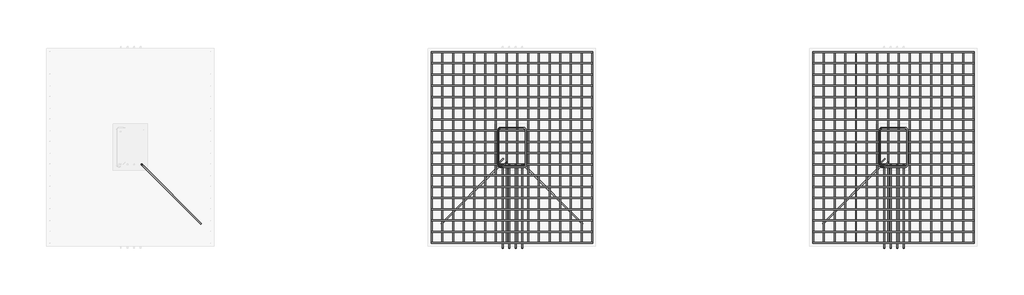
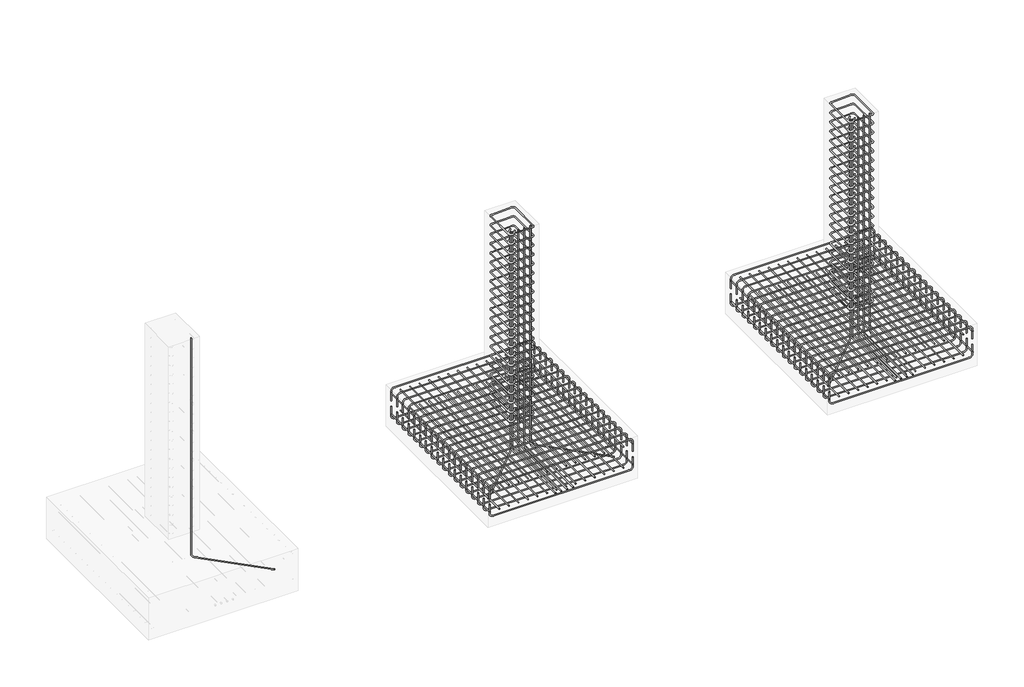
# One storey, part 7 of 33: 16 reinforcing bars.
"""IFC4 building model written with IfcOpenShell, lengths in millimetres."""

from ifc_helpers import new_model, si_unit, point, frame, origin, place, context, project, spatial, polyline, circle_curve, trimmed, segment, composite_curve, source, transform, mapped, element, save
from ifc_brep_helpers import swept_disk

model = new_model("IFC4")

# Units and contexts
model_context = context("Model", 3, world=origin())
ifc_project = project(units=[si_unit("LENGTHUNIT", "METRE", prefix="MILLI")], contexts=[model_context])

# Site, building, storey
site = spatial("IfcSite", under=ifc_project)
building = spatial("IfcBuilding", under=site)
storey = spatial("IfcBuildingStorey", under=building, Elevation=-3000.0)

# Reinforcing bars
placement = place(None, origin())
reinforcing_bar_shape = source(origin(), model_context, "Body", "SolidModel", [
    swept_disk(composite_curve([segment(polyline([(9306.5357258, -7044.0608134, -3240.0), (9306.5357258, -7044.0608134, -3092.7)]), True, "CONTINUOUS"), segment(trimmed(circle_curve(frame((9352.8857258, -7044.0608134, -3092.7), z_axis=(0.0, 1.0, 0.0), x_axis=(-46.350000000000364, 0.0, 0.0)), 46.35), [point((9306.5357258, -7044.0608134, -3092.7))], [point((9352.8857258, -7044.0608134, -3046.35))], True, "CARTESIAN"), True, "CONTINUOUS"), segment(polyline([(9352.8857258, -7044.0608134, -3046.35), (11367.4857258, -7044.0608134, -3046.35)]), True, "CONTINUOUS"), segment(trimmed(circle_curve(frame((11367.4857258, -7044.0608134, -3092.7), z_axis=(0.0, 1.0, 0.0), x_axis=(0.0, 0.0, 46.34999999999991)), 46.35), [point((11367.4857258, -7044.0608134, -3046.35))], [point((11413.8357258, -7044.0608134, -3092.7))], True, "CARTESIAN"), True, "CONTINUOUS"), segment(polyline([(11413.8357258, -7044.0608134, -3092.7), (11413.8357258, -7044.0608134, -3240.0)]), True, "CONTINUOUS")], self_intersect=False), 6.35),
])
element("IfcReinforcingBar", 1, at=placement, inside=storey, context=model_context, shape_type="MappedRepresentation", body=[
    mapped(reinforcing_bar_shape, transform((0.0, 0.0, 0.0), x_axis=(1.0, 0.0, 0.0), y_axis=(0.0, 1.0, 0.0), z_axis=(0.0, 0.0, 1.0))),
    mapped(reinforcing_bar_shape, transform((0.0, -147.4882353, 0.0), x_axis=(1.0, 0.0, 0.0), y_axis=(0.0, 1.0, 0.0), z_axis=(0.0, 0.0, 1.0))),
    mapped(reinforcing_bar_shape, transform((0.0, -294.9764706, 0.0), x_axis=(1.0, 0.0, 0.0), y_axis=(0.0, 1.0, 0.0), z_axis=(0.0, 0.0, 1.0))),
    mapped(reinforcing_bar_shape, transform((0.0, -442.4647059, 0.0), x_axis=(1.0, 0.0, 0.0), y_axis=(0.0, 1.0, 0.0), z_axis=(0.0, 0.0, 1.0))),
    mapped(reinforcing_bar_shape, transform((0.0, -589.9529412, 0.0), x_axis=(1.0, 0.0, 0.0), y_axis=(0.0, 1.0, 0.0), z_axis=(0.0, 0.0, 1.0))),
    mapped(reinforcing_bar_shape, transform((0.0, -737.4411765, 0.0), x_axis=(1.0, 0.0, 0.0), y_axis=(0.0, 1.0, 0.0), z_axis=(0.0, 0.0, 1.0))),
    mapped(reinforcing_bar_shape, transform((0.0, -884.9294118, 0.0), x_axis=(1.0, 0.0, 0.0), y_axis=(0.0, 1.0, 0.0), z_axis=(0.0, 0.0, 1.0))),
    mapped(reinforcing_bar_shape, transform((0.0, -1032.4176471, 0.0), x_axis=(1.0, 0.0, 0.0), y_axis=(0.0, 1.0, 0.0), z_axis=(0.0, 0.0, 1.0))),
    mapped(reinforcing_bar_shape, transform((0.0, -1179.9058824, 0.0), x_axis=(1.0, 0.0, 0.0), y_axis=(0.0, 1.0, 0.0), z_axis=(0.0, 0.0, 1.0))),
    mapped(reinforcing_bar_shape, transform((0.0, -1327.3941176, 0.0), x_axis=(1.0, 0.0, 0.0), y_axis=(0.0, 1.0, 0.0), z_axis=(0.0, 0.0, 1.0))),
    mapped(reinforcing_bar_shape, transform((0.0, -1474.8823529, 0.0), x_axis=(1.0, 0.0, 0.0), y_axis=(0.0, 1.0, 0.0), z_axis=(0.0, 0.0, 1.0))),
    mapped(reinforcing_bar_shape, transform((0.0, -1622.3705882, 0.0), x_axis=(1.0, 0.0, 0.0), y_axis=(0.0, 1.0, 0.0), z_axis=(0.0, 0.0, 1.0))),
    mapped(reinforcing_bar_shape, transform((0.0, -1769.8588235, 0.0), x_axis=(1.0, 0.0, 0.0), y_axis=(0.0, 1.0, 0.0), z_axis=(0.0, 0.0, 1.0))),
    mapped(reinforcing_bar_shape, transform((0.0, -1917.3470588, 0.0), x_axis=(1.0, 0.0, 0.0), y_axis=(0.0, 1.0, 0.0), z_axis=(0.0, 0.0, 1.0))),
    mapped(reinforcing_bar_shape, transform((0.0, -2064.8352941, 0.0), x_axis=(1.0, 0.0, 0.0), y_axis=(0.0, 1.0, 0.0), z_axis=(0.0, 0.0, 1.0))),
    mapped(reinforcing_bar_shape, transform((0.0, -2212.3235294, 0.0), x_axis=(1.0, 0.0, 0.0), y_axis=(0.0, 1.0, 0.0), z_axis=(0.0, 0.0, 1.0))),
    mapped(reinforcing_bar_shape, transform((0.0, -2359.8117647, 0.0), x_axis=(1.0, 0.0, 0.0), y_axis=(0.0, 1.0, 0.0), z_axis=(0.0, 0.0, 1.0))),
    mapped(reinforcing_bar_shape, transform((0.0, -2507.3, 0.0), x_axis=(1.0, 0.0, 0.0), y_axis=(0.0, 1.0, 0.0), z_axis=(0.0, 0.0, 1.0))),
])
reinforcing_bar_2_shape = source(origin(), model_context, "Body", "SolidModel", [
    swept_disk(composite_curve([segment(polyline([(11413.8357258, -7044.0608134, -3330.080452), (11413.8357258, -7044.0608134, -3477.380452)]), True, "CONTINUOUS"), segment(trimmed(circle_curve(frame((11367.4857258, -7044.0608134, -3477.380452), z_axis=(0.0, 1.0, 0.0), x_axis=(46.350000000000364, 0.0, 0.0)), 46.35), [point((11413.8357258, -7044.0608134, -3477.380452))], [point((11367.4857258, -7044.0608134, -3523.730452))], True, "CARTESIAN"), True, "CONTINUOUS"), segment(polyline([(11367.4857258, -7044.0608134, -3523.730452), (9352.8857258, -7044.0608134, -3523.730452)]), True, "CONTINUOUS"), segment(trimmed(circle_curve(frame((9352.8857258, -7044.0608134, -3477.380452), z_axis=(0.0, 1.0, 0.0), x_axis=(0.0, 0.0, -46.34999999999991)), 46.35), [point((9352.8857258, -7044.0608134, -3523.730452))], [point((9306.5357258, -7044.0608134, -3477.380452))], True, "CARTESIAN"), True, "CONTINUOUS"), segment(polyline([(9306.5357258, -7044.0608134, -3477.380452), (9306.5357258, -7044.0608134, -3330.080452)]), True, "CONTINUOUS")], self_intersect=False), 6.35),
])
element("IfcReinforcingBar", 2, at=placement, inside=storey, context=model_context, shape_type="MappedRepresentation", body=[
    mapped(reinforcing_bar_2_shape, transform((0.0, 0.0, 0.0), x_axis=(1.0, 0.0, 0.0), y_axis=(0.0, 1.0, 0.0), z_axis=(0.0, 0.0, 1.0))),
    mapped(reinforcing_bar_2_shape, transform((0.0, -147.4882353, 0.0), x_axis=(1.0, 0.0, 0.0), y_axis=(0.0, 1.0, 0.0), z_axis=(0.0, 0.0, 1.0))),
    mapped(reinforcing_bar_2_shape, transform((0.0, -294.9764706, 0.0), x_axis=(1.0, 0.0, 0.0), y_axis=(0.0, 1.0, 0.0), z_axis=(0.0, 0.0, 1.0))),
    mapped(reinforcing_bar_2_shape, transform((0.0, -442.4647059, 0.0), x_axis=(1.0, 0.0, 0.0), y_axis=(0.0, 1.0, 0.0), z_axis=(0.0, 0.0, 1.0))),
    mapped(reinforcing_bar_2_shape, transform((0.0, -589.9529412, 0.0), x_axis=(1.0, 0.0, 0.0), y_axis=(0.0, 1.0, 0.0), z_axis=(0.0, 0.0, 1.0))),
    mapped(reinforcing_bar_2_shape, transform((0.0, -737.4411765, 0.0), x_axis=(1.0, 0.0, 0.0), y_axis=(0.0, 1.0, 0.0), z_axis=(0.0, 0.0, 1.0))),
    mapped(reinforcing_bar_2_shape, transform((0.0, -884.9294118, 0.0), x_axis=(1.0, 0.0, 0.0), y_axis=(0.0, 1.0, 0.0), z_axis=(0.0, 0.0, 1.0))),
    mapped(reinforcing_bar_2_shape, transform((0.0, -1032.4176471, 0.0), x_axis=(1.0, 0.0, 0.0), y_axis=(0.0, 1.0, 0.0), z_axis=(0.0, 0.0, 1.0))),
    mapped(reinforcing_bar_2_shape, transform((0.0, -1179.9058824, 0.0), x_axis=(1.0, 0.0, 0.0), y_axis=(0.0, 1.0, 0.0), z_axis=(0.0, 0.0, 1.0))),
    mapped(reinforcing_bar_2_shape, transform((0.0, -1327.3941176, 0.0), x_axis=(1.0, 0.0, 0.0), y_axis=(0.0, 1.0, 0.0), z_axis=(0.0, 0.0, 1.0))),
    mapped(reinforcing_bar_2_shape, transform((0.0, -1474.8823529, 0.0), x_axis=(1.0, 0.0, 0.0), y_axis=(0.0, 1.0, 0.0), z_axis=(0.0, 0.0, 1.0))),
    mapped(reinforcing_bar_2_shape, transform((0.0, -1622.3705882, 0.0), x_axis=(1.0, 0.0, 0.0), y_axis=(0.0, 1.0, 0.0), z_axis=(0.0, 0.0, 1.0))),
    mapped(reinforcing_bar_2_shape, transform((0.0, -1769.8588235, 0.0), x_axis=(1.0, 0.0, 0.0), y_axis=(0.0, 1.0, 0.0), z_axis=(0.0, 0.0, 1.0))),
    mapped(reinforcing_bar_2_shape, transform((0.0, -1917.3470588, 0.0), x_axis=(1.0, 0.0, 0.0), y_axis=(0.0, 1.0, 0.0), z_axis=(0.0, 0.0, 1.0))),
    mapped(reinforcing_bar_2_shape, transform((0.0, -2064.8352941, 0.0), x_axis=(1.0, 0.0, 0.0), y_axis=(0.0, 1.0, 0.0), z_axis=(0.0, 0.0, 1.0))),
    mapped(reinforcing_bar_2_shape, transform((0.0, -2212.3235294, 0.0), x_axis=(1.0, 0.0, 0.0), y_axis=(0.0, 1.0, 0.0), z_axis=(0.0, 0.0, 1.0))),
    mapped(reinforcing_bar_2_shape, transform((0.0, -2359.8117647, 0.0), x_axis=(1.0, 0.0, 0.0), y_axis=(0.0, 1.0, 0.0), z_axis=(0.0, 0.0, 1.0))),
    mapped(reinforcing_bar_2_shape, transform((0.0, -2507.3, 0.0), x_axis=(1.0, 0.0, 0.0), y_axis=(0.0, 1.0, 0.0), z_axis=(0.0, 0.0, 1.0))),
])
reinforcing_bar_3_shape = source(origin(), model_context, "Body", "SolidModel", [
    swept_disk(composite_curve([segment(polyline([(11413.8357258, -9557.7108134, -3447.8614173), (11413.8357258, -7037.7108134, -3447.8614173)]), True, "CONTINUOUS")], self_intersect=False), 6.35),
])
element("IfcReinforcingBar", 3, at=placement, inside=storey, context=model_context, shape_type="MappedRepresentation", body=[
    mapped(reinforcing_bar_3_shape, transform((0.0, 0.0, 0.0), x_axis=(1.0, 0.0, 0.0), y_axis=(0.0, 1.0, 0.0), z_axis=(0.0, 0.0, 1.0))),
    mapped(reinforcing_bar_3_shape, transform((-140.4866667, 0.0, 0.0), x_axis=(1.0, 0.0, 0.0), y_axis=(0.0, 1.0, 0.0), z_axis=(0.0, 0.0, 1.0))),
    mapped(reinforcing_bar_3_shape, transform((-280.9733333, 0.0, 0.0), x_axis=(1.0, 0.0, 0.0), y_axis=(0.0, 1.0, 0.0), z_axis=(0.0, 0.0, 1.0))),
    mapped(reinforcing_bar_3_shape, transform((-421.46, 0.0, 0.0), x_axis=(1.0, 0.0, 0.0), y_axis=(0.0, 1.0, 0.0), z_axis=(0.0, 0.0, 1.0))),
    mapped(reinforcing_bar_3_shape, transform((-561.9466667, 0.0, 0.0), x_axis=(1.0, 0.0, 0.0), y_axis=(0.0, 1.0, 0.0), z_axis=(0.0, 0.0, 1.0))),
    mapped(reinforcing_bar_3_shape, transform((-702.4333333, 0.0, 0.0), x_axis=(1.0, 0.0, 0.0), y_axis=(0.0, 1.0, 0.0), z_axis=(0.0, 0.0, 1.0))),
    mapped(reinforcing_bar_3_shape, transform((-842.92, 0.0, 0.0), x_axis=(1.0, 0.0, 0.0), y_axis=(0.0, 1.0, 0.0), z_axis=(0.0, 0.0, 1.0))),
    mapped(reinforcing_bar_3_shape, transform((-983.4066667, 0.0, 0.0), x_axis=(1.0, 0.0, 0.0), y_axis=(0.0, 1.0, 0.0), z_axis=(0.0, 0.0, 1.0))),
    mapped(reinforcing_bar_3_shape, transform((-1123.8933333, 0.0, 0.0), x_axis=(1.0, 0.0, 0.0), y_axis=(0.0, 1.0, 0.0), z_axis=(0.0, 0.0, 1.0))),
    mapped(reinforcing_bar_3_shape, transform((-1264.38, 0.0, 0.0), x_axis=(1.0, 0.0, 0.0), y_axis=(0.0, 1.0, 0.0), z_axis=(0.0, 0.0, 1.0))),
    mapped(reinforcing_bar_3_shape, transform((-1404.8666667, 0.0, 0.0), x_axis=(1.0, 0.0, 0.0), y_axis=(0.0, 1.0, 0.0), z_axis=(0.0, 0.0, 1.0))),
    mapped(reinforcing_bar_3_shape, transform((-1545.3533333, 0.0, 0.0), x_axis=(1.0, 0.0, 0.0), y_axis=(0.0, 1.0, 0.0), z_axis=(0.0, 0.0, 1.0))),
    mapped(reinforcing_bar_3_shape, transform((-1685.84, 0.0, 0.0), x_axis=(1.0, 0.0, 0.0), y_axis=(0.0, 1.0, 0.0), z_axis=(0.0, 0.0, 1.0))),
    mapped(reinforcing_bar_3_shape, transform((-1826.3266667, 0.0, 0.0), x_axis=(1.0, 0.0, 0.0), y_axis=(0.0, 1.0, 0.0), z_axis=(0.0, 0.0, 1.0))),
    mapped(reinforcing_bar_3_shape, transform((-1966.8133333, 0.0, 0.0), x_axis=(1.0, 0.0, 0.0), y_axis=(0.0, 1.0, 0.0), z_axis=(0.0, 0.0, 1.0))),
    mapped(reinforcing_bar_3_shape, transform((-2107.3, 0.0, 0.0), x_axis=(1.0, 0.0, 0.0), y_axis=(0.0, 1.0, 0.0), z_axis=(0.0, 0.0, 1.0))),
])
reinforcing_bar_4_shape = source(origin(), model_context, "Body", "SolidModel", [
    swept_disk(composite_curve([segment(polyline([(9306.5357258, -9557.7108134, -3122.7084113), (9306.5357258, -7037.7108134, -3122.7084113)]), True, "CONTINUOUS")], self_intersect=False), 6.35),
])
element("IfcReinforcingBar", 4, at=placement, inside=storey, context=model_context, shape_type="MappedRepresentation", body=[
    mapped(reinforcing_bar_4_shape, transform((0.0, 0.0, 0.0), x_axis=(1.0, 0.0, 0.0), y_axis=(0.0, 1.0, 0.0), z_axis=(0.0, 0.0, 1.0))),
    mapped(reinforcing_bar_4_shape, transform((140.4866667, 0.0, 0.0), x_axis=(1.0, 0.0, 0.0), y_axis=(0.0, 1.0, 0.0), z_axis=(0.0, 0.0, 1.0))),
    mapped(reinforcing_bar_4_shape, transform((280.9733333, 0.0, 0.0), x_axis=(1.0, 0.0, 0.0), y_axis=(0.0, 1.0, 0.0), z_axis=(0.0, 0.0, 1.0))),
    mapped(reinforcing_bar_4_shape, transform((421.46, 0.0, 0.0), x_axis=(1.0, 0.0, 0.0), y_axis=(0.0, 1.0, 0.0), z_axis=(0.0, 0.0, 1.0))),
    mapped(reinforcing_bar_4_shape, transform((561.9466667, 0.0, 0.0), x_axis=(1.0, 0.0, 0.0), y_axis=(0.0, 1.0, 0.0), z_axis=(0.0, 0.0, 1.0))),
    mapped(reinforcing_bar_4_shape, transform((702.4333333, 0.0, 0.0), x_axis=(1.0, 0.0, 0.0), y_axis=(0.0, 1.0, 0.0), z_axis=(0.0, 0.0, 1.0))),
    mapped(reinforcing_bar_4_shape, transform((842.92, 0.0, 0.0), x_axis=(1.0, 0.0, 0.0), y_axis=(0.0, 1.0, 0.0), z_axis=(0.0, 0.0, 1.0))),
    mapped(reinforcing_bar_4_shape, transform((983.4066667, 0.0, 0.0), x_axis=(1.0, 0.0, 0.0), y_axis=(0.0, 1.0, 0.0), z_axis=(0.0, 0.0, 1.0))),
    mapped(reinforcing_bar_4_shape, transform((1123.8933333, 0.0, 0.0), x_axis=(1.0, 0.0, 0.0), y_axis=(0.0, 1.0, 0.0), z_axis=(0.0, 0.0, 1.0))),
    mapped(reinforcing_bar_4_shape, transform((1264.38, 0.0, 0.0), x_axis=(1.0, 0.0, 0.0), y_axis=(0.0, 1.0, 0.0), z_axis=(0.0, 0.0, 1.0))),
    mapped(reinforcing_bar_4_shape, transform((1404.8666667, 0.0, 0.0), x_axis=(1.0, 0.0, 0.0), y_axis=(0.0, 1.0, 0.0), z_axis=(0.0, 0.0, 1.0))),
    mapped(reinforcing_bar_4_shape, transform((1545.3533333, 0.0, 0.0), x_axis=(1.0, 0.0, 0.0), y_axis=(0.0, 1.0, 0.0), z_axis=(0.0, 0.0, 1.0))),
    mapped(reinforcing_bar_4_shape, transform((1685.84, 0.0, 0.0), x_axis=(1.0, 0.0, 0.0), y_axis=(0.0, 1.0, 0.0), z_axis=(0.0, 0.0, 1.0))),
    mapped(reinforcing_bar_4_shape, transform((1826.3266667, 0.0, 0.0), x_axis=(1.0, 0.0, 0.0), y_axis=(0.0, 1.0, 0.0), z_axis=(0.0, 0.0, 1.0))),
    mapped(reinforcing_bar_4_shape, transform((1966.8133333, 0.0, 0.0), x_axis=(1.0, 0.0, 0.0), y_axis=(0.0, 1.0, 0.0), z_axis=(0.0, 0.0, 1.0))),
    mapped(reinforcing_bar_4_shape, transform((2107.3, 0.0, 0.0), x_axis=(1.0, 0.0, 0.0), y_axis=(0.0, 1.0, 0.0), z_axis=(0.0, 0.0, 1.0))),
])
reinforcing_bar_5_shape = source(origin(), model_context, "Body", "SolidModel", [
    swept_disk(composite_curve([segment(polyline([(4306.5357258, -7044.0608134, -3240.0), (4306.5357258, -7044.0608134, -3092.7)]), True, "CONTINUOUS"), segment(trimmed(circle_curve(frame((4352.8857258, -7044.0608134, -3092.7), z_axis=(0.0, 1.0, 0.0), x_axis=(-46.349999999999454, 0.0, 0.0)), 46.35), [point((4306.5357258, -7044.0608134, -3092.7))], [point((4352.8857258, -7044.0608134, -3046.35))], True, "CARTESIAN"), True, "CONTINUOUS"), segment(polyline([(4352.8857258, -7044.0608134, -3046.35), (6367.4857258, -7044.0608134, -3046.35)]), True, "CONTINUOUS"), segment(trimmed(circle_curve(frame((6367.4857258, -7044.0608134, -3092.7), z_axis=(0.0, 1.0, 0.0), x_axis=(0.0, 0.0, 46.34999999999991)), 46.35), [point((6367.4857258, -7044.0608134, -3046.35))], [point((6413.8357258, -7044.0608134, -3092.7))], True, "CARTESIAN"), True, "CONTINUOUS"), segment(polyline([(6413.8357258, -7044.0608134, -3092.7), (6413.8357258, -7044.0608134, -3240.0)]), True, "CONTINUOUS")], self_intersect=False), 6.35),
])
element("IfcReinforcingBar", 5, at=placement, inside=storey, context=model_context, shape_type="MappedRepresentation", body=[
    mapped(reinforcing_bar_5_shape, transform((0.0, 0.0, 0.0), x_axis=(1.0, 0.0, 0.0), y_axis=(0.0, 1.0, 0.0), z_axis=(0.0, 0.0, 1.0))),
    mapped(reinforcing_bar_5_shape, transform((0.0, -147.4882353, 0.0), x_axis=(1.0, 0.0, 0.0), y_axis=(0.0, 1.0, 0.0), z_axis=(0.0, 0.0, 1.0))),
    mapped(reinforcing_bar_5_shape, transform((0.0, -294.9764706, 0.0), x_axis=(1.0, 0.0, 0.0), y_axis=(0.0, 1.0, 0.0), z_axis=(0.0, 0.0, 1.0))),
    mapped(reinforcing_bar_5_shape, transform((0.0, -442.4647059, 0.0), x_axis=(1.0, 0.0, 0.0), y_axis=(0.0, 1.0, 0.0), z_axis=(0.0, 0.0, 1.0))),
    mapped(reinforcing_bar_5_shape, transform((0.0, -589.9529412, 0.0), x_axis=(1.0, 0.0, 0.0), y_axis=(0.0, 1.0, 0.0), z_axis=(0.0, 0.0, 1.0))),
    mapped(reinforcing_bar_5_shape, transform((0.0, -737.4411765, 0.0), x_axis=(1.0, 0.0, 0.0), y_axis=(0.0, 1.0, 0.0), z_axis=(0.0, 0.0, 1.0))),
    mapped(reinforcing_bar_5_shape, transform((0.0, -884.9294118, 0.0), x_axis=(1.0, 0.0, 0.0), y_axis=(0.0, 1.0, 0.0), z_axis=(0.0, 0.0, 1.0))),
    mapped(reinforcing_bar_5_shape, transform((0.0, -1032.4176471, 0.0), x_axis=(1.0, 0.0, 0.0), y_axis=(0.0, 1.0, 0.0), z_axis=(0.0, 0.0, 1.0))),
    mapped(reinforcing_bar_5_shape, transform((0.0, -1179.9058824, 0.0), x_axis=(1.0, 0.0, 0.0), y_axis=(0.0, 1.0, 0.0), z_axis=(0.0, 0.0, 1.0))),
    mapped(reinforcing_bar_5_shape, transform((0.0, -1327.3941176, 0.0), x_axis=(1.0, 0.0, 0.0), y_axis=(0.0, 1.0, 0.0), z_axis=(0.0, 0.0, 1.0))),
    mapped(reinforcing_bar_5_shape, transform((0.0, -1474.8823529, 0.0), x_axis=(1.0, 0.0, 0.0), y_axis=(0.0, 1.0, 0.0), z_axis=(0.0, 0.0, 1.0))),
    mapped(reinforcing_bar_5_shape, transform((0.0, -1622.3705882, 0.0), x_axis=(1.0, 0.0, 0.0), y_axis=(0.0, 1.0, 0.0), z_axis=(0.0, 0.0, 1.0))),
    mapped(reinforcing_bar_5_shape, transform((0.0, -1769.8588235, 0.0), x_axis=(1.0, 0.0, 0.0), y_axis=(0.0, 1.0, 0.0), z_axis=(0.0, 0.0, 1.0))),
    mapped(reinforcing_bar_5_shape, transform((0.0, -1917.3470588, 0.0), x_axis=(1.0, 0.0, 0.0), y_axis=(0.0, 1.0, 0.0), z_axis=(0.0, 0.0, 1.0))),
    mapped(reinforcing_bar_5_shape, transform((0.0, -2064.8352941, 0.0), x_axis=(1.0, 0.0, 0.0), y_axis=(0.0, 1.0, 0.0), z_axis=(0.0, 0.0, 1.0))),
    mapped(reinforcing_bar_5_shape, transform((0.0, -2212.3235294, 0.0), x_axis=(1.0, 0.0, 0.0), y_axis=(0.0, 1.0, 0.0), z_axis=(0.0, 0.0, 1.0))),
    mapped(reinforcing_bar_5_shape, transform((0.0, -2359.8117647, 0.0), x_axis=(1.0, 0.0, 0.0), y_axis=(0.0, 1.0, 0.0), z_axis=(0.0, 0.0, 1.0))),
    mapped(reinforcing_bar_5_shape, transform((0.0, -2507.3, 0.0), x_axis=(1.0, 0.0, 0.0), y_axis=(0.0, 1.0, 0.0), z_axis=(0.0, 0.0, 1.0))),
])
reinforcing_bar_6_shape = source(origin(), model_context, "Body", "SolidModel", [
    swept_disk(composite_curve([segment(polyline([(6413.8357258, -7044.0608134, -3330.080452), (6413.8357258, -7044.0608134, -3477.380452)]), True, "CONTINUOUS"), segment(trimmed(circle_curve(frame((6367.4857258, -7044.0608134, -3477.380452), z_axis=(0.0, 1.0, 0.0), x_axis=(46.349999999999454, 0.0, 0.0)), 46.35), [point((6413.8357258, -7044.0608134, -3477.380452))], [point((6367.4857258, -7044.0608134, -3523.730452))], True, "CARTESIAN"), True, "CONTINUOUS"), segment(polyline([(6367.4857258, -7044.0608134, -3523.730452), (4352.8857258, -7044.0608134, -3523.730452)]), True, "CONTINUOUS"), segment(trimmed(circle_curve(frame((4352.8857258, -7044.0608134, -3477.380452), z_axis=(0.0, 1.0, 0.0), x_axis=(0.0, 0.0, -46.34999999999991)), 46.35), [point((4352.8857258, -7044.0608134, -3523.730452))], [point((4306.5357258, -7044.0608134, -3477.380452))], True, "CARTESIAN"), True, "CONTINUOUS"), segment(polyline([(4306.5357258, -7044.0608134, -3477.380452), (4306.5357258, -7044.0608134, -3330.080452)]), True, "CONTINUOUS")], self_intersect=False), 6.35),
])
element("IfcReinforcingBar", 6, at=placement, inside=storey, context=model_context, shape_type="MappedRepresentation", body=[
    mapped(reinforcing_bar_6_shape, transform((0.0, 0.0, 0.0), x_axis=(1.0, 0.0, 0.0), y_axis=(0.0, 1.0, 0.0), z_axis=(0.0, 0.0, 1.0))),
    mapped(reinforcing_bar_6_shape, transform((0.0, -147.4882353, 0.0), x_axis=(1.0, 0.0, 0.0), y_axis=(0.0, 1.0, 0.0), z_axis=(0.0, 0.0, 1.0))),
    mapped(reinforcing_bar_6_shape, transform((0.0, -294.9764706, 0.0), x_axis=(1.0, 0.0, 0.0), y_axis=(0.0, 1.0, 0.0), z_axis=(0.0, 0.0, 1.0))),
    mapped(reinforcing_bar_6_shape, transform((0.0, -442.4647059, 0.0), x_axis=(1.0, 0.0, 0.0), y_axis=(0.0, 1.0, 0.0), z_axis=(0.0, 0.0, 1.0))),
    mapped(reinforcing_bar_6_shape, transform((0.0, -589.9529412, 0.0), x_axis=(1.0, 0.0, 0.0), y_axis=(0.0, 1.0, 0.0), z_axis=(0.0, 0.0, 1.0))),
    mapped(reinforcing_bar_6_shape, transform((0.0, -737.4411765, 0.0), x_axis=(1.0, 0.0, 0.0), y_axis=(0.0, 1.0, 0.0), z_axis=(0.0, 0.0, 1.0))),
    mapped(reinforcing_bar_6_shape, transform((0.0, -884.9294118, 0.0), x_axis=(1.0, 0.0, 0.0), y_axis=(0.0, 1.0, 0.0), z_axis=(0.0, 0.0, 1.0))),
    mapped(reinforcing_bar_6_shape, transform((0.0, -1032.4176471, 0.0), x_axis=(1.0, 0.0, 0.0), y_axis=(0.0, 1.0, 0.0), z_axis=(0.0, 0.0, 1.0))),
    mapped(reinforcing_bar_6_shape, transform((0.0, -1179.9058824, 0.0), x_axis=(1.0, 0.0, 0.0), y_axis=(0.0, 1.0, 0.0), z_axis=(0.0, 0.0, 1.0))),
    mapped(reinforcing_bar_6_shape, transform((0.0, -1327.3941176, 0.0), x_axis=(1.0, 0.0, 0.0), y_axis=(0.0, 1.0, 0.0), z_axis=(0.0, 0.0, 1.0))),
    mapped(reinforcing_bar_6_shape, transform((0.0, -1474.8823529, 0.0), x_axis=(1.0, 0.0, 0.0), y_axis=(0.0, 1.0, 0.0), z_axis=(0.0, 0.0, 1.0))),
    mapped(reinforcing_bar_6_shape, transform((0.0, -1622.3705882, 0.0), x_axis=(1.0, 0.0, 0.0), y_axis=(0.0, 1.0, 0.0), z_axis=(0.0, 0.0, 1.0))),
    mapped(reinforcing_bar_6_shape, transform((0.0, -1769.8588235, 0.0), x_axis=(1.0, 0.0, 0.0), y_axis=(0.0, 1.0, 0.0), z_axis=(0.0, 0.0, 1.0))),
    mapped(reinforcing_bar_6_shape, transform((0.0, -1917.3470588, 0.0), x_axis=(1.0, 0.0, 0.0), y_axis=(0.0, 1.0, 0.0), z_axis=(0.0, 0.0, 1.0))),
    mapped(reinforcing_bar_6_shape, transform((0.0, -2064.8352941, 0.0), x_axis=(1.0, 0.0, 0.0), y_axis=(0.0, 1.0, 0.0), z_axis=(0.0, 0.0, 1.0))),
    mapped(reinforcing_bar_6_shape, transform((0.0, -2212.3235294, 0.0), x_axis=(1.0, 0.0, 0.0), y_axis=(0.0, 1.0, 0.0), z_axis=(0.0, 0.0, 1.0))),
    mapped(reinforcing_bar_6_shape, transform((0.0, -2359.8117647, 0.0), x_axis=(1.0, 0.0, 0.0), y_axis=(0.0, 1.0, 0.0), z_axis=(0.0, 0.0, 1.0))),
    mapped(reinforcing_bar_6_shape, transform((0.0, -2507.3, 0.0), x_axis=(1.0, 0.0, 0.0), y_axis=(0.0, 1.0, 0.0), z_axis=(0.0, 0.0, 1.0))),
])
reinforcing_bar_7_shape = source(origin(), model_context, "Body", "SolidModel", [
    swept_disk(composite_curve([segment(polyline([(6413.8357258, -9557.7108134, -3447.8614173), (6413.8357258, -7037.7108134, -3447.8614173)]), True, "CONTINUOUS")], self_intersect=False), 6.35),
])
element("IfcReinforcingBar", 7, at=placement, inside=storey, context=model_context, shape_type="MappedRepresentation", body=[
    mapped(reinforcing_bar_7_shape, transform((0.0, 0.0, 0.0), x_axis=(1.0, 0.0, 0.0), y_axis=(0.0, 1.0, 0.0), z_axis=(0.0, 0.0, 1.0))),
    mapped(reinforcing_bar_7_shape, transform((-140.4866667, 0.0, 0.0), x_axis=(1.0, 0.0, 0.0), y_axis=(0.0, 1.0, 0.0), z_axis=(0.0, 0.0, 1.0))),
    mapped(reinforcing_bar_7_shape, transform((-280.9733333, 0.0, 0.0), x_axis=(1.0, 0.0, 0.0), y_axis=(0.0, 1.0, 0.0), z_axis=(0.0, 0.0, 1.0))),
    mapped(reinforcing_bar_7_shape, transform((-421.46, 0.0, 0.0), x_axis=(1.0, 0.0, 0.0), y_axis=(0.0, 1.0, 0.0), z_axis=(0.0, 0.0, 1.0))),
    mapped(reinforcing_bar_7_shape, transform((-561.9466667, 0.0, 0.0), x_axis=(1.0, 0.0, 0.0), y_axis=(0.0, 1.0, 0.0), z_axis=(0.0, 0.0, 1.0))),
    mapped(reinforcing_bar_7_shape, transform((-702.4333333, 0.0, 0.0), x_axis=(1.0, 0.0, 0.0), y_axis=(0.0, 1.0, 0.0), z_axis=(0.0, 0.0, 1.0))),
    mapped(reinforcing_bar_7_shape, transform((-842.92, 0.0, 0.0), x_axis=(1.0, 0.0, 0.0), y_axis=(0.0, 1.0, 0.0), z_axis=(0.0, 0.0, 1.0))),
    mapped(reinforcing_bar_7_shape, transform((-983.4066667, 0.0, 0.0), x_axis=(1.0, 0.0, 0.0), y_axis=(0.0, 1.0, 0.0), z_axis=(0.0, 0.0, 1.0))),
    mapped(reinforcing_bar_7_shape, transform((-1123.8933333, 0.0, 0.0), x_axis=(1.0, 0.0, 0.0), y_axis=(0.0, 1.0, 0.0), z_axis=(0.0, 0.0, 1.0))),
    mapped(reinforcing_bar_7_shape, transform((-1264.38, 0.0, 0.0), x_axis=(1.0, 0.0, 0.0), y_axis=(0.0, 1.0, 0.0), z_axis=(0.0, 0.0, 1.0))),
    mapped(reinforcing_bar_7_shape, transform((-1404.8666667, 0.0, 0.0), x_axis=(1.0, 0.0, 0.0), y_axis=(0.0, 1.0, 0.0), z_axis=(0.0, 0.0, 1.0))),
    mapped(reinforcing_bar_7_shape, transform((-1545.3533333, 0.0, 0.0), x_axis=(1.0, 0.0, 0.0), y_axis=(0.0, 1.0, 0.0), z_axis=(0.0, 0.0, 1.0))),
    mapped(reinforcing_bar_7_shape, transform((-1685.84, 0.0, 0.0), x_axis=(1.0, 0.0, 0.0), y_axis=(0.0, 1.0, 0.0), z_axis=(0.0, 0.0, 1.0))),
    mapped(reinforcing_bar_7_shape, transform((-1826.3266667, 0.0, 0.0), x_axis=(1.0, 0.0, 0.0), y_axis=(0.0, 1.0, 0.0), z_axis=(0.0, 0.0, 1.0))),
    mapped(reinforcing_bar_7_shape, transform((-1966.8133333, 0.0, 0.0), x_axis=(1.0, 0.0, 0.0), y_axis=(0.0, 1.0, 0.0), z_axis=(0.0, 0.0, 1.0))),
    mapped(reinforcing_bar_7_shape, transform((-2107.3, 0.0, 0.0), x_axis=(1.0, 0.0, 0.0), y_axis=(0.0, 1.0, 0.0), z_axis=(0.0, 0.0, 1.0))),
])
reinforcing_bar_8_shape = source(origin(), model_context, "Body", "SolidModel", [
    swept_disk(composite_curve([segment(polyline([(4306.5357258, -9557.7108134, -3122.7084113), (4306.5357258, -7037.7108134, -3122.7084113)]), True, "CONTINUOUS")], self_intersect=False), 6.35),
])
element("IfcReinforcingBar", 8, at=placement, inside=storey, context=model_context, shape_type="MappedRepresentation", body=[
    mapped(reinforcing_bar_8_shape, transform((0.0, 0.0, 0.0), x_axis=(1.0, 0.0, 0.0), y_axis=(0.0, 1.0, 0.0), z_axis=(0.0, 0.0, 1.0))),
    mapped(reinforcing_bar_8_shape, transform((140.4866667, 0.0, 0.0), x_axis=(1.0, 0.0, 0.0), y_axis=(0.0, 1.0, 0.0), z_axis=(0.0, 0.0, 1.0))),
    mapped(reinforcing_bar_8_shape, transform((280.9733333, 0.0, 0.0), x_axis=(1.0, 0.0, 0.0), y_axis=(0.0, 1.0, 0.0), z_axis=(0.0, 0.0, 1.0))),
    mapped(reinforcing_bar_8_shape, transform((421.46, 0.0, 0.0), x_axis=(1.0, 0.0, 0.0), y_axis=(0.0, 1.0, 0.0), z_axis=(0.0, 0.0, 1.0))),
    mapped(reinforcing_bar_8_shape, transform((561.9466667, 0.0, 0.0), x_axis=(1.0, 0.0, 0.0), y_axis=(0.0, 1.0, 0.0), z_axis=(0.0, 0.0, 1.0))),
    mapped(reinforcing_bar_8_shape, transform((702.4333333, 0.0, 0.0), x_axis=(1.0, 0.0, 0.0), y_axis=(0.0, 1.0, 0.0), z_axis=(0.0, 0.0, 1.0))),
    mapped(reinforcing_bar_8_shape, transform((842.92, 0.0, 0.0), x_axis=(1.0, 0.0, 0.0), y_axis=(0.0, 1.0, 0.0), z_axis=(0.0, 0.0, 1.0))),
    mapped(reinforcing_bar_8_shape, transform((983.4066667, 0.0, 0.0), x_axis=(1.0, 0.0, 0.0), y_axis=(0.0, 1.0, 0.0), z_axis=(0.0, 0.0, 1.0))),
    mapped(reinforcing_bar_8_shape, transform((1123.8933333, 0.0, 0.0), x_axis=(1.0, 0.0, 0.0), y_axis=(0.0, 1.0, 0.0), z_axis=(0.0, 0.0, 1.0))),
    mapped(reinforcing_bar_8_shape, transform((1264.38, 0.0, 0.0), x_axis=(1.0, 0.0, 0.0), y_axis=(0.0, 1.0, 0.0), z_axis=(0.0, 0.0, 1.0))),
    mapped(reinforcing_bar_8_shape, transform((1404.8666667, 0.0, 0.0), x_axis=(1.0, 0.0, 0.0), y_axis=(0.0, 1.0, 0.0), z_axis=(0.0, 0.0, 1.0))),
    mapped(reinforcing_bar_8_shape, transform((1545.3533333, 0.0, 0.0), x_axis=(1.0, 0.0, 0.0), y_axis=(0.0, 1.0, 0.0), z_axis=(0.0, 0.0, 1.0))),
    mapped(reinforcing_bar_8_shape, transform((1685.84, 0.0, 0.0), x_axis=(1.0, 0.0, 0.0), y_axis=(0.0, 1.0, 0.0), z_axis=(0.0, 0.0, 1.0))),
    mapped(reinforcing_bar_8_shape, transform((1826.3266667, 0.0, 0.0), x_axis=(1.0, 0.0, 0.0), y_axis=(0.0, 1.0, 0.0), z_axis=(0.0, 0.0, 1.0))),
    mapped(reinforcing_bar_8_shape, transform((1966.8133333, 0.0, 0.0), x_axis=(1.0, 0.0, 0.0), y_axis=(0.0, 1.0, 0.0), z_axis=(0.0, 0.0, 1.0))),
    mapped(reinforcing_bar_8_shape, transform((2107.3, 0.0, 0.0), x_axis=(1.0, 0.0, 0.0), y_axis=(0.0, 1.0, 0.0), z_axis=(0.0, 0.0, 1.0))),
])
element("IfcReinforcingBar", 9, at=placement, inside=storey, context=model_context, shape_type="SolidModel", body=[
    swept_disk(composite_curve([segment(polyline([(507.1671301, -8521.6339414, -40.0), (507.1671301, -8521.6339414, -3393.65)]), True, "CONTINUOUS"), segment(trimmed(circle_curve(frame((539.9415294, -8554.4083407, -3393.65), z_axis=(-0.7071067811865493, -0.7071067811865459, 0.0), x_axis=(-32.77439930000003, 32.77439930000037, 0.0)), 46.35), [point((507.1671301, -8521.6339414, -3393.65))], [point((539.9415294, -8554.4083407, -3440.0))], True, "CARTESIAN"), True, "CONTINUOUS"), segment(polyline([(539.9415294, -8554.4083407, -3440.0), (1284.9845894, -9299.4514007, -3440.0)]), True, "CONTINUOUS")], self_intersect=False), 6.35),
])
reinforcing_bar_9_shape = source(origin(), model_context, "Body", "SolidModel", [
    swept_disk(composite_curve([segment(polyline([(5246.4614911, -8446.8994528, -2953.65), (5190.7179282, -8502.6430158, -2953.65)]), True, "CONTINUOUS"), segment(trimmed(circle_curve(frame((5212.8857258, -8524.8108134, -2953.65), z_axis=(0.0, 0.0, 1.0), x_axis=(-22.167797600000085, 22.167797599999176, 0.0)), 31.35), [point((5190.7179282, -8502.6430158, -2953.65))], [point((5212.8857258, -8556.1608134, -2953.65))], True, "CARTESIAN"), True, "CONTINUOUS"), segment(polyline([(5212.8857258, -8556.1608134, -2953.65), (5507.4857258, -8556.1608134, -2953.65)]), True, "CONTINUOUS"), segment(trimmed(circle_curve(frame((5507.4857258, -8524.8108134, -2953.65), z_axis=(0.0, 0.0, 1.0), x_axis=(0.0, -31.350000000000364, 0.0)), 31.35), [point((5507.4857258, -8556.1608134, -2953.65))], [point((5538.8357258, -8524.8108134, -2953.65))], True, "CARTESIAN"), True, "CONTINUOUS"), segment(polyline([(5538.8357258, -8524.8108134, -2953.65), (5538.8357258, -8070.6108134, -2953.65)]), True, "CONTINUOUS"), segment(trimmed(circle_curve(frame((5507.5055109, -8070.6108134, -2954.7636125), z_axis=(-0.0355219283344822, 0.0, 0.9993688971583016), x_axis=(31.33021489999919, 0.0, 1.1136124999998174)), 31.35), [point((5538.8357258, -8070.6108134, -2953.65))], [point((5507.5055109, -8039.2608134, -2954.7636125))], True, "CARTESIAN"), True, "CONTINUOUS"), segment(polyline([(5507.5055109, -8039.2608134, -2954.7636125), (5212.8659407, -8039.2608134, -2965.2363875)]), True, "CONTINUOUS"), segment(trimmed(circle_curve(frame((5212.8659407, -8070.6108134, -2965.2363875), z_axis=(-0.0355219283344822, 0.0, 0.9993688971583016), x_axis=(0.0, 31.349999999999454, 0.0)), 31.35), [point((5212.8659407, -8039.2608134, -2965.2363875))], [point((5181.5357258, -8070.6108134, -2966.35))], True, "CARTESIAN"), True, "CONTINUOUS"), segment(polyline([(5181.5357258, -8070.6108134, -2966.35), (5181.5357258, -8524.8108134, -2966.35)]), True, "CONTINUOUS"), segment(trimmed(circle_curve(frame((5212.8857258, -8524.8108134, -2966.35), z_axis=(0.0, 0.0, 1.0), x_axis=(-31.349999999999454, 0.0, 0.0)), 31.35), [point((5181.5357258, -8524.8108134, -2966.35))], [point((5235.0535234, -8546.978611, -2966.35))], True, "CARTESIAN"), True, "CONTINUOUS"), segment(polyline([(5235.0535234, -8546.978611, -2966.35), (5290.7970863, -8491.235048, -2966.35)]), True, "CONTINUOUS")], self_intersect=False), 6.35),
])
element("IfcReinforcingBar", 10, at=placement, inside=storey, context=model_context, shape_type="MappedRepresentation", body=[
    mapped(reinforcing_bar_9_shape, transform((0.0, 0.0, 0.0), x_axis=(1.0, 0.0, 0.0), y_axis=(0.0, 1.0, 0.0), z_axis=(0.0, 0.0, 1.0))),
    mapped(reinforcing_bar_9_shape, transform((0.0, 0.0, 145.365), x_axis=(1.0, 0.0, 0.0), y_axis=(0.0, 1.0, 0.0), z_axis=(0.0, 0.0, 1.0))),
    mapped(reinforcing_bar_9_shape, transform((0.0, 0.0, 290.73), x_axis=(1.0, 0.0, 0.0), y_axis=(0.0, 1.0, 0.0), z_axis=(0.0, 0.0, 1.0))),
    mapped(reinforcing_bar_9_shape, transform((0.0, 0.0, 436.095), x_axis=(1.0, 0.0, 0.0), y_axis=(0.0, 1.0, 0.0), z_axis=(0.0, 0.0, 1.0))),
    mapped(reinforcing_bar_9_shape, transform((0.0, 0.0, 581.46), x_axis=(1.0, 0.0, 0.0), y_axis=(0.0, 1.0, 0.0), z_axis=(0.0, 0.0, 1.0))),
    mapped(reinforcing_bar_9_shape, transform((0.0, 0.0, 726.825), x_axis=(1.0, 0.0, 0.0), y_axis=(0.0, 1.0, 0.0), z_axis=(0.0, 0.0, 1.0))),
    mapped(reinforcing_bar_9_shape, transform((0.0, 0.0, 872.19), x_axis=(1.0, 0.0, 0.0), y_axis=(0.0, 1.0, 0.0), z_axis=(0.0, 0.0, 1.0))),
    mapped(reinforcing_bar_9_shape, transform((0.0, 0.0, 1017.555), x_axis=(1.0, 0.0, 0.0), y_axis=(0.0, 1.0, 0.0), z_axis=(0.0, 0.0, 1.0))),
    mapped(reinforcing_bar_9_shape, transform((0.0, 0.0, 1162.92), x_axis=(1.0, 0.0, 0.0), y_axis=(0.0, 1.0, 0.0), z_axis=(0.0, 0.0, 1.0))),
    mapped(reinforcing_bar_9_shape, transform((0.0, 0.0, 1308.285), x_axis=(1.0, 0.0, 0.0), y_axis=(0.0, 1.0, 0.0), z_axis=(0.0, 0.0, 1.0))),
    mapped(reinforcing_bar_9_shape, transform((0.0, 0.0, 1453.65), x_axis=(1.0, 0.0, 0.0), y_axis=(0.0, 1.0, 0.0), z_axis=(0.0, 0.0, 1.0))),
    mapped(reinforcing_bar_9_shape, transform((0.0, 0.0, 1599.015), x_axis=(1.0, 0.0, 0.0), y_axis=(0.0, 1.0, 0.0), z_axis=(0.0, 0.0, 1.0))),
    mapped(reinforcing_bar_9_shape, transform((0.0, 0.0, 1744.38), x_axis=(1.0, 0.0, 0.0), y_axis=(0.0, 1.0, 0.0), z_axis=(0.0, 0.0, 1.0))),
    mapped(reinforcing_bar_9_shape, transform((0.0, 0.0, 1889.745), x_axis=(1.0, 0.0, 0.0), y_axis=(0.0, 1.0, 0.0), z_axis=(0.0, 0.0, 1.0))),
    mapped(reinforcing_bar_9_shape, transform((0.0, 0.0, 2035.11), x_axis=(1.0, 0.0, 0.0), y_axis=(0.0, 1.0, 0.0), z_axis=(0.0, 0.0, 1.0))),
    mapped(reinforcing_bar_9_shape, transform((0.0, 0.0, 2180.475), x_axis=(1.0, 0.0, 0.0), y_axis=(0.0, 1.0, 0.0), z_axis=(0.0, 0.0, 1.0))),
    mapped(reinforcing_bar_9_shape, transform((0.0, 0.0, 2325.84), x_axis=(1.0, 0.0, 0.0), y_axis=(0.0, 1.0, 0.0), z_axis=(0.0, 0.0, 1.0))),
    mapped(reinforcing_bar_9_shape, transform((0.0, 0.0, 2471.205), x_axis=(1.0, 0.0, 0.0), y_axis=(0.0, 1.0, 0.0), z_axis=(0.0, 0.0, 1.0))),
    mapped(reinforcing_bar_9_shape, transform((0.0, 0.0, 2616.57), x_axis=(1.0, 0.0, 0.0), y_axis=(0.0, 1.0, 0.0), z_axis=(0.0, 0.0, 1.0))),
    mapped(reinforcing_bar_9_shape, transform((0.0, 0.0, 2761.935), x_axis=(1.0, 0.0, 0.0), y_axis=(0.0, 1.0, 0.0), z_axis=(0.0, 0.0, 1.0))),
    mapped(reinforcing_bar_9_shape, transform((0.0, 0.0, 2907.3), x_axis=(1.0, 0.0, 0.0), y_axis=(0.0, 1.0, 0.0), z_axis=(0.0, 0.0, 1.0))),
])
element("IfcReinforcingBar", 11, at=placement, inside=storey, context=model_context, shape_type="SolidModel", body=[
    swept_disk(composite_curve([segment(polyline([(5213.2043214, -8521.6339414, -40.0), (5213.2043214, -8521.6339414, -3393.65)]), True, "CONTINUOUS"), segment(trimmed(circle_curve(frame((5180.4299221, -8554.4083407, -3393.65), z_axis=(-0.7071067811865446, 0.7071067811865505, 0.0), x_axis=(32.77439929999946, 32.77439930000037, 0.0)), 46.35), [point((5213.2043214, -8521.6339414, -3393.65))], [point((5180.4299221, -8554.4083407, -3440.0))], True, "CARTESIAN"), True, "CONTINUOUS"), segment(polyline([(5180.4299221, -8554.4083407, -3440.0), (4435.3868621, -9299.4514007, -3440.0)]), True, "CONTINUOUS")], self_intersect=False), 6.35),
])
element("IfcReinforcingBar", 12, at=placement, inside=storey, context=model_context, shape_type="SolidModel", body=[
    swept_disk(composite_curve([segment(polyline([(5507.1671301, -8521.6339414, -40.0), (5507.1671301, -8521.6339414, -3393.65)]), True, "CONTINUOUS"), segment(trimmed(circle_curve(frame((5539.9415294, -8554.4083407, -3393.65), z_axis=(-0.7071067811865493, -0.7071067811865459, 0.0), x_axis=(-32.77439930000037, 32.77439930000037, 0.0)), 46.35), [point((5507.1671301, -8521.6339414, -3393.65))], [point((5539.9415294, -8554.4083407, -3440.0))], True, "CARTESIAN"), True, "CONTINUOUS"), segment(polyline([(5539.9415294, -8554.4083407, -3440.0), (6284.9845894, -9299.4514007, -3440.0)]), True, "CONTINUOUS")], self_intersect=False), 6.35),
])
reinforcing_bar_10_shape = source(origin(), model_context, "Body", "SolidModel", [
    swept_disk(composite_curve([segment(polyline([(5236.1158322, -8523.4938134, -40.0), (5236.1158322, -8523.4938134, -3393.65)]), True, "CONTINUOUS"), segment(trimmed(circle_curve(frame((5236.1158322, -8569.8438134, -3393.65), z_axis=(-1.0, 0.0, 0.0), x_axis=(0.0, 46.350000000000364, 0.0)), 46.35), [point((5236.1158322, -8523.4938134, -3393.65))], [point((5236.1158322, -8569.8438134, -3440.0))], True, "CARTESIAN"), True, "CONTINUOUS"), segment(polyline([(5236.1158322, -8569.8438134, -3440.0), (5236.1158322, -9623.4938134, -3440.0)]), True, "CONTINUOUS")], self_intersect=False), 6.35),
])
element("IfcReinforcingBar", 13, at=placement, inside=storey, context=model_context, shape_type="MappedRepresentation", body=[
    mapped(reinforcing_bar_10_shape, transform((0.0, 0.0, 0.0), x_axis=(1.0, 0.0, 0.0), y_axis=(0.0, 1.0, 0.0), z_axis=(0.0, 0.0, 1.0))),
    mapped(reinforcing_bar_10_shape, transform((86.8979716, 0.0, 0.0), x_axis=(1.0, 0.0, 0.0), y_axis=(0.0, 1.0, 0.0), z_axis=(0.0, 0.0, 1.0))),
    mapped(reinforcing_bar_10_shape, transform((173.7959432, 0.0, 0.0), x_axis=(1.0, 0.0, 0.0), y_axis=(0.0, 1.0, 0.0), z_axis=(0.0, 0.0, 1.0))),
    mapped(reinforcing_bar_10_shape, transform((260.6939148, 0.0, 0.0), x_axis=(1.0, 0.0, 0.0), y_axis=(0.0, 1.0, 0.0), z_axis=(0.0, 0.0, 1.0))),
])
reinforcing_bar_11_shape = source(origin(), model_context, "Body", "SolidModel", [
    swept_disk(composite_curve([segment(polyline([(10246.4614911, -8446.8994528, -2953.65), (10190.7179282, -8502.6430158, -2953.65)]), True, "CONTINUOUS"), segment(trimmed(circle_curve(frame((10212.8857258, -8524.8108134, -2953.65), z_axis=(0.0, 0.0, 1.0), x_axis=(-22.167797600000995, 22.167797599999176, 0.0)), 31.35), [point((10190.7179282, -8502.6430158, -2953.65))], [point((10212.8857258, -8556.1608134, -2953.65))], True, "CARTESIAN"), True, "CONTINUOUS"), segment(polyline([(10212.8857258, -8556.1608134, -2953.65), (10507.4857258, -8556.1608134, -2953.65)]), True, "CONTINUOUS"), segment(trimmed(circle_curve(frame((10507.4857258, -8524.8108134, -2953.65), z_axis=(0.0, 0.0, 1.0), x_axis=(0.0, -31.350000000000364, 0.0)), 31.35), [point((10507.4857258, -8556.1608134, -2953.65))], [point((10538.8357258, -8524.8108134, -2953.65))], True, "CARTESIAN"), True, "CONTINUOUS"), segment(polyline([(10538.8357258, -8524.8108134, -2953.65), (10538.8357258, -8070.6108134, -2953.65)]), True, "CONTINUOUS"), segment(trimmed(circle_curve(frame((10507.5055109, -8070.6108134, -2954.7636125), z_axis=(-0.0355219283344822, 0.0, 0.9993688971583016), x_axis=(31.33021489999919, 0.0, 1.1136124999998174)), 31.35), [point((10538.8357258, -8070.6108134, -2953.65))], [point((10507.5055109, -8039.2608134, -2954.7636125))], True, "CARTESIAN"), True, "CONTINUOUS"), segment(polyline([(10507.5055109, -8039.2608134, -2954.7636125), (10212.8659407, -8039.2608134, -2965.2363875)]), True, "CONTINUOUS"), segment(trimmed(circle_curve(frame((10212.8659407, -8070.6108134, -2965.2363875), z_axis=(-0.0355219283344822, 0.0, 0.9993688971583016), x_axis=(0.0, 31.349999999999454, 0.0)), 31.35), [point((10212.8659407, -8039.2608134, -2965.2363875))], [point((10181.5357258, -8070.6108134, -2966.35))], True, "CARTESIAN"), True, "CONTINUOUS"), segment(polyline([(10181.5357258, -8070.6108134, -2966.35), (10181.5357258, -8524.8108134, -2966.35)]), True, "CONTINUOUS"), segment(trimmed(circle_curve(frame((10212.8857258, -8524.8108134, -2966.35), z_axis=(0.0, 0.0, 1.0), x_axis=(-31.350000000000364, 0.0, 0.0)), 31.35), [point((10181.5357258, -8524.8108134, -2966.35))], [point((10235.0535234, -8546.978611, -2966.35))], True, "CARTESIAN"), True, "CONTINUOUS"), segment(polyline([(10235.0535234, -8546.978611, -2966.35), (10290.7970863, -8491.235048, -2966.35)]), True, "CONTINUOUS")], self_intersect=False), 6.35),
])
element("IfcReinforcingBar", 14, at=placement, inside=storey, context=model_context, shape_type="MappedRepresentation", body=[
    mapped(reinforcing_bar_11_shape, transform((0.0, 0.0, 0.0), x_axis=(1.0, 0.0, 0.0), y_axis=(0.0, 1.0, 0.0), z_axis=(0.0, 0.0, 1.0))),
    mapped(reinforcing_bar_11_shape, transform((0.0, 0.0, 145.365), x_axis=(1.0, 0.0, 0.0), y_axis=(0.0, 1.0, 0.0), z_axis=(0.0, 0.0, 1.0))),
    mapped(reinforcing_bar_11_shape, transform((0.0, 0.0, 290.73), x_axis=(1.0, 0.0, 0.0), y_axis=(0.0, 1.0, 0.0), z_axis=(0.0, 0.0, 1.0))),
    mapped(reinforcing_bar_11_shape, transform((0.0, 0.0, 436.095), x_axis=(1.0, 0.0, 0.0), y_axis=(0.0, 1.0, 0.0), z_axis=(0.0, 0.0, 1.0))),
    mapped(reinforcing_bar_11_shape, transform((0.0, 0.0, 581.46), x_axis=(1.0, 0.0, 0.0), y_axis=(0.0, 1.0, 0.0), z_axis=(0.0, 0.0, 1.0))),
    mapped(reinforcing_bar_11_shape, transform((0.0, 0.0, 726.825), x_axis=(1.0, 0.0, 0.0), y_axis=(0.0, 1.0, 0.0), z_axis=(0.0, 0.0, 1.0))),
    mapped(reinforcing_bar_11_shape, transform((0.0, 0.0, 872.19), x_axis=(1.0, 0.0, 0.0), y_axis=(0.0, 1.0, 0.0), z_axis=(0.0, 0.0, 1.0))),
    mapped(reinforcing_bar_11_shape, transform((0.0, 0.0, 1017.555), x_axis=(1.0, 0.0, 0.0), y_axis=(0.0, 1.0, 0.0), z_axis=(0.0, 0.0, 1.0))),
    mapped(reinforcing_bar_11_shape, transform((0.0, 0.0, 1162.92), x_axis=(1.0, 0.0, 0.0), y_axis=(0.0, 1.0, 0.0), z_axis=(0.0, 0.0, 1.0))),
    mapped(reinforcing_bar_11_shape, transform((0.0, 0.0, 1308.285), x_axis=(1.0, 0.0, 0.0), y_axis=(0.0, 1.0, 0.0), z_axis=(0.0, 0.0, 1.0))),
    mapped(reinforcing_bar_11_shape, transform((0.0, 0.0, 1453.65), x_axis=(1.0, 0.0, 0.0), y_axis=(0.0, 1.0, 0.0), z_axis=(0.0, 0.0, 1.0))),
    mapped(reinforcing_bar_11_shape, transform((0.0, 0.0, 1599.015), x_axis=(1.0, 0.0, 0.0), y_axis=(0.0, 1.0, 0.0), z_axis=(0.0, 0.0, 1.0))),
    mapped(reinforcing_bar_11_shape, transform((0.0, 0.0, 1744.38), x_axis=(1.0, 0.0, 0.0), y_axis=(0.0, 1.0, 0.0), z_axis=(0.0, 0.0, 1.0))),
    mapped(reinforcing_bar_11_shape, transform((0.0, 0.0, 1889.745), x_axis=(1.0, 0.0, 0.0), y_axis=(0.0, 1.0, 0.0), z_axis=(0.0, 0.0, 1.0))),
    mapped(reinforcing_bar_11_shape, transform((0.0, 0.0, 2035.11), x_axis=(1.0, 0.0, 0.0), y_axis=(0.0, 1.0, 0.0), z_axis=(0.0, 0.0, 1.0))),
    mapped(reinforcing_bar_11_shape, transform((0.0, 0.0, 2180.475), x_axis=(1.0, 0.0, 0.0), y_axis=(0.0, 1.0, 0.0), z_axis=(0.0, 0.0, 1.0))),
    mapped(reinforcing_bar_11_shape, transform((0.0, 0.0, 2325.84), x_axis=(1.0, 0.0, 0.0), y_axis=(0.0, 1.0, 0.0), z_axis=(0.0, 0.0, 1.0))),
    mapped(reinforcing_bar_11_shape, transform((0.0, 0.0, 2471.205), x_axis=(1.0, 0.0, 0.0), y_axis=(0.0, 1.0, 0.0), z_axis=(0.0, 0.0, 1.0))),
    mapped(reinforcing_bar_11_shape, transform((0.0, 0.0, 2616.57), x_axis=(1.0, 0.0, 0.0), y_axis=(0.0, 1.0, 0.0), z_axis=(0.0, 0.0, 1.0))),
    mapped(reinforcing_bar_11_shape, transform((0.0, 0.0, 2761.935), x_axis=(1.0, 0.0, 0.0), y_axis=(0.0, 1.0, 0.0), z_axis=(0.0, 0.0, 1.0))),
    mapped(reinforcing_bar_11_shape, transform((0.0, 0.0, 2907.3), x_axis=(1.0, 0.0, 0.0), y_axis=(0.0, 1.0, 0.0), z_axis=(0.0, 0.0, 1.0))),
])
element("IfcReinforcingBar", 15, at=placement, inside=storey, context=model_context, shape_type="SolidModel", body=[
    swept_disk(composite_curve([segment(polyline([(10213.2043214, -8521.6339414, -40.0), (10213.2043214, -8521.6339414, -3393.65)]), True, "CONTINUOUS"), segment(trimmed(circle_curve(frame((10180.4299221, -8554.4083407, -3393.65), z_axis=(-0.7071067811865446, 0.7071067811865505, 0.0), x_axis=(32.77439930000037, 32.77439930000037, 0.0)), 46.35), [point((10213.2043214, -8521.6339414, -3393.65))], [point((10180.4299221, -8554.4083407, -3440.0))], True, "CARTESIAN"), True, "CONTINUOUS"), segment(polyline([(10180.4299221, -8554.4083407, -3440.0), (9435.3868621, -9299.4514007, -3440.0)]), True, "CONTINUOUS")], self_intersect=False), 6.35),
])
reinforcing_bar_12_shape = source(origin(), model_context, "Body", "SolidModel", [
    swept_disk(composite_curve([segment(polyline([(10236.1158322, -8523.4938134, -40.0), (10236.1158322, -8523.4938134, -3393.65)]), True, "CONTINUOUS"), segment(trimmed(circle_curve(frame((10236.1158322, -8569.8438134, -3393.65), z_axis=(-1.0, 0.0, 0.0), x_axis=(0.0, 46.350000000000364, 0.0)), 46.35), [point((10236.1158322, -8523.4938134, -3393.65))], [point((10236.1158322, -8569.8438134, -3440.0))], True, "CARTESIAN"), True, "CONTINUOUS"), segment(polyline([(10236.1158322, -8569.8438134, -3440.0), (10236.1158322, -9623.4938134, -3440.0)]), True, "CONTINUOUS")], self_intersect=False), 6.35),
])
element("IfcReinforcingBar", 16, at=placement, inside=storey, context=model_context, shape_type="MappedRepresentation", body=[
    mapped(reinforcing_bar_12_shape, transform((0.0, 0.0, 0.0), x_axis=(1.0, 0.0, 0.0), y_axis=(0.0, 1.0, 0.0), z_axis=(0.0, 0.0, 1.0))),
    mapped(reinforcing_bar_12_shape, transform((86.8979716, 0.0, 0.0), x_axis=(1.0, 0.0, 0.0), y_axis=(0.0, 1.0, 0.0), z_axis=(0.0, 0.0, 1.0))),
    mapped(reinforcing_bar_12_shape, transform((173.7959432, 0.0, 0.0), x_axis=(1.0, 0.0, 0.0), y_axis=(0.0, 1.0, 0.0), z_axis=(0.0, 0.0, 1.0))),
    mapped(reinforcing_bar_12_shape, transform((260.6939148, 0.0, 0.0), x_axis=(1.0, 0.0, 0.0), y_axis=(0.0, 1.0, 0.0), z_axis=(0.0, 0.0, 1.0))),
])

save(model, "model.ifc")

# Revit data of these elements
# Elements 1, 2, 3, 4, 5, 6, 7, 8, 9, 10, 11, 12, 13, 14, 15, 16 (IfcReinforcingBar)
#   Phase Created = New Construction
